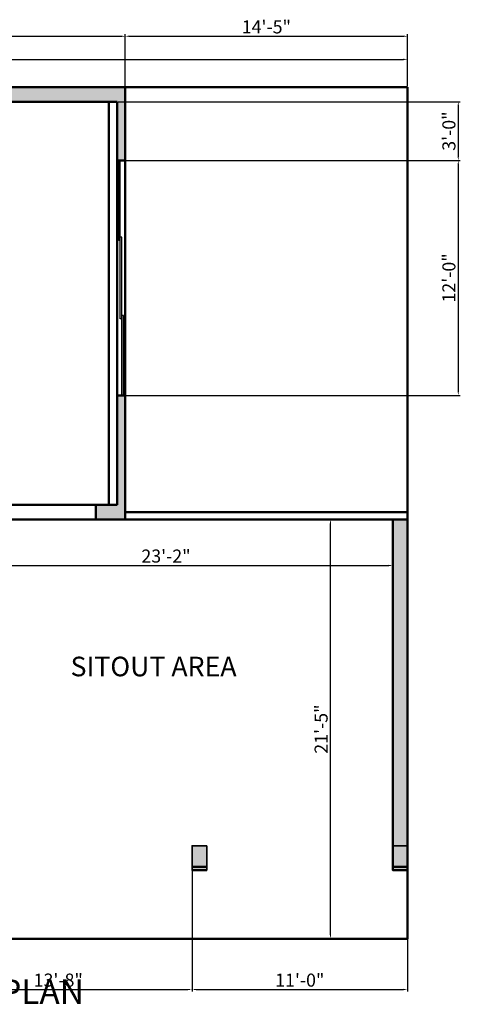
# Model space of a CAD drawing. Units: inches. Extents: x 1770 to 3141, y 984 to 1614.
# Tile 12 of 12: x 2871 to 3141, y 1003 to 1606. Entities that reach past the tile are written whole.
import ezdxf

# ---------------------------------------------------------------- set-up
doc = ezdxf.new("R2010")
doc.units = ezdxf.units.IN
for name, color, linetype, lineweight in [('A-ANNO-DIMS', 2, 'Continuous', 18), ('A-ANNO-TEXT', 7, 'Continuous', 18), ('A-AREA-IDEN', 3, 'Continuous', 18), ('A-COLS', 1, 'Continuous', 35), ('A-GLAZ', 5, 'Continuous', 25), ('A-WALL', 7, 'Continuous', 50), ('A-WALL-PATT', 8, 'Continuous', 13)]:
    doc.layers.add(name, color=color, linetype=linetype, lineweight=lineweight)
doc.styles.get("Standard").update_dxf_attribs({"font": 'arial.ttf'})
doc.dimstyles.new('ISO-25', dxfattribs={"dimtxt": 8, "dimasz": 2.5, "dimexe": 1.25, "dimexo": 0.625, "dimtad": 1, "dimdec": 1, "dimlunit": 3, "dimtxsty": 'Standard', "dimcen": 2.5, "dimclrt": 1, "dimadec": 0, "dimazin": 0, "dimtfac": 1, "dimtdec": 1, "dimtmove": 0, "dimatfit": 3, "dimfxl": 1, "dimarcsym": 0})

# ---------------------------------------------------------------- blocks, each defined once
blk = doc.blocks.new('*D20')
at = {"layer": 'A-ANNO-DIMS', "color": 0, "lineweight": -2, "transparency": 16777216}
for p, q in [((2509.08, 1565.8), (2509.08, 1583.37)), ((2511.58, 1582.12), (3106.58, 1582.12)), ((3109.08, 1565.8), (3109.08, 1583.37))]:
    blk.add_line(p, q, dxfattribs=at)
at = {"layer": 'A-ANNO-DIMS', "color": 0, "transparency": 16777216}
for points in [[(2511.58, 1582.54), (2511.58, 1581.7), (2509.08, 1582.12)], [(3106.58, 1582.54), (3106.58, 1581.7), (3109.08, 1582.12)]]:
    blk.add_solid(points, dxfattribs=at)
at = {"layer": 'Defpoints', "color": 0, "transparency": 16777216}
for p in [(3109.08, 1582.12), (2509.08, 1565.18), (3109.08, 1565.18)]:
    blk.add_point(p, dxfattribs=at)
at = {"layer": 'A-ANNO-DIMS', "color": 0, "transparency": 16777216, "insert": (2809.08, 1586.83), "char_height": 8, "attachment_point": 5}
blk.add_mtext("50'", dxfattribs=at)
blk = doc.blocks.new('*D52')
at = {"layer": 'A-ANNO-DIMS', "color": 0, "lineweight": -2, "transparency": 16777216}
for p, q in [((2822.08, 1274.4), (2822.08, 1270.71)), ((3100.08, 1274.4), (3100.08, 1270.71)), ((2824.58, 1271.96), (3097.58, 1271.96))]:
    blk.add_line(p, q, dxfattribs=at)
at = {"layer": 'A-ANNO-DIMS', "color": 0, "transparency": 16777216}
for points in [[(2824.58, 1272.38), (2824.58, 1271.54), (2822.08, 1271.96)], [(3097.58, 1272.38), (3097.58, 1271.54), (3100.08, 1271.96)]]:
    blk.add_solid(points, dxfattribs=at)
at = {"layer": 'Defpoints', "color": 0, "transparency": 16777216}
for p in [(2822.08, 1275.03), (3100.08, 1275.03), (3100.08, 1271.96)]:
    blk.add_point(p, dxfattribs=at)
at = {"layer": 'A-ANNO-DIMS', "color": 0, "transparency": 16777216, "insert": (2961.08, 1276.67), "char_height": 8, "attachment_point": 5}
blk.add_mtext('23\'-2"', dxfattribs=at)
blk = doc.blocks.new('*D53')
at = {"layer": 'A-ANNO-DIMS', "color": 0, "lineweight": -2, "transparency": 16777216}
for p, q in [((3061.88, 1045.68), (3061.88, 1297.68)), ((3062.5, 1300.18), (3063.13, 1300.18)), ((3062.5, 1043.18), (3063.13, 1043.18))]:
    blk.add_line(p, q, dxfattribs=at)
at = {"layer": 'A-ANNO-DIMS', "color": 0, "transparency": 16777216}
for points in [[(3061.46, 1297.68), (3062.29, 1297.68), (3061.88, 1300.18)], [(3061.46, 1045.68), (3062.29, 1045.68), (3061.88, 1043.18)]]:
    blk.add_solid(points, dxfattribs=at)
at = {"layer": 'Defpoints', "color": 0, "transparency": 16777216}
for p in [(3061.88, 1300.18), (3061.88, 1300.18), (3061.88, 1043.18)]:
    blk.add_point(p, dxfattribs=at)
at = {"layer": 'A-ANNO-DIMS', "color": 0, "transparency": 16777216, "insert": (3057.17, 1171.68), "char_height": 8, "attachment_point": 5, "rotation": 90}
blk.add_mtext('21\'-5"', dxfattribs=at)
blk = doc.blocks.new('COLUMN-9x15')
at = {"transparency": 33554687}
h = blk.add_hatch(color=256, dxfattribs=at)
h.dxf.hatch_style = 1
h.paths.add_polyline_path([(9, 15), (0, 15), (0, 0), (9, 0)])
blk.add_lwpolyline([(9, 15), (0, 15), (0, 0), (9, 0)], close=True)
blk = doc.blocks.new('*D124')
at = {"layer": 'A-ANNO-DIMS', "color": 0, "lineweight": -2, "transparency": 16777216}
for p, q in [((2735.08, 1556.8), (2735.08, 1597.53)), ((2737.58, 1596.28), (2933.58, 1596.28)), ((2936.08, 1565.8), (2936.08, 1597.53))]:
    blk.add_line(p, q, dxfattribs=at)
at = {"layer": 'A-ANNO-DIMS', "color": 0, "transparency": 16777216}
for points in [[(2737.58, 1596.7), (2737.58, 1595.86), (2735.08, 1596.28)], [(2933.58, 1596.7), (2933.58, 1595.86), (2936.08, 1596.28)]]:
    blk.add_solid(points, dxfattribs=at)
at = {"layer": 'Defpoints', "color": 0, "transparency": 16777216}
for p in [(2936.08, 1596.28), (2936.08, 1565.18), (2735.08, 1556.18)]:
    blk.add_point(p, dxfattribs=at)
at = {"layer": 'A-ANNO-DIMS', "color": 1, "transparency": 16777216, "insert": (2835.58, 1600.99), "char_height": 8, "attachment_point": 5}
blk.add_mtext('16\'-9"', dxfattribs=at)
blk = doc.blocks.new('*D125')
at = {"layer": 'A-ANNO-DIMS', "color": 0, "lineweight": -2, "transparency": 16777216}
for p, q in [((2936.08, 1565.8), (2936.08, 1597.53)), ((2938.58, 1596.28), (3106.58, 1596.28)), ((3109.08, 1565.8), (3109.08, 1597.53))]:
    blk.add_line(p, q, dxfattribs=at)
at = {"layer": 'A-ANNO-DIMS', "color": 0, "transparency": 16777216}
for points in [[(2938.58, 1596.7), (2938.58, 1595.86), (2936.08, 1596.28)], [(3106.58, 1596.7), (3106.58, 1595.86), (3109.08, 1596.28)]]:
    blk.add_solid(points, dxfattribs=at)
at = {"layer": 'Defpoints', "color": 0, "transparency": 16777216}
for p in [(3109.08, 1596.28), (2936.08, 1565.18), (3109.08, 1565.18)]:
    blk.add_point(p, dxfattribs=at)
at = {"layer": 'A-ANNO-DIMS', "color": 1, "transparency": 16777216, "insert": (3022.58, 1600.99), "char_height": 8, "attachment_point": 5}
blk.add_mtext('14\'-5"', dxfattribs=at)
blk = doc.blocks.new('*D133')
at = {"layer": 'A-ANNO-DIMS', "color": 0, "lineweight": -2, "transparency": 16777216}
for p, q in [((2813.08, 1084.55), (2813.08, 1010.83)), ((2977.04, 1084.55), (2977.04, 1010.83)), ((2815.58, 1012.08), (2974.54, 1012.08))]:
    blk.add_line(p, q, dxfattribs=at)
at = {"layer": 'A-ANNO-DIMS', "color": 0, "transparency": 16777216}
for points in [[(2815.58, 1012.5), (2815.58, 1011.66), (2813.08, 1012.08)], [(2974.54, 1012.5), (2974.54, 1011.66), (2977.04, 1012.08)]]:
    blk.add_solid(points, dxfattribs=at)
at = {"layer": 'Defpoints', "color": 0, "transparency": 16777216}
for p in [(2813.08, 1085.18), (2977.04, 1085.18), (2977.04, 1012.08)]:
    blk.add_point(p, dxfattribs=at)
at = {"layer": 'A-ANNO-DIMS', "color": 1, "transparency": 16777216, "insert": (2895.06, 1016.79), "char_height": 8, "attachment_point": 5}
blk.add_mtext('13\'-8"', dxfattribs=at)
blk = doc.blocks.new('*D134')
at = {"layer": 'A-ANNO-DIMS', "color": 0, "lineweight": -2, "transparency": 16777216}
for p, q in [((2977.04, 1084.55), (2977.04, 1010.83)), ((3109.08, 1084.55), (3109.08, 1010.83)), ((2979.54, 1012.08), (3106.58, 1012.08))]:
    blk.add_line(p, q, dxfattribs=at)
at = {"layer": 'A-ANNO-DIMS', "color": 0, "transparency": 16777216}
for points in [[(2979.54, 1012.5), (2979.54, 1011.66), (2977.04, 1012.08)], [(3106.58, 1012.5), (3106.58, 1011.66), (3109.08, 1012.08)]]:
    blk.add_solid(points, dxfattribs=at)
at = {"layer": 'Defpoints', "color": 0, "transparency": 16777216}
for p in [(2977.04, 1085.18), (3109.08, 1085.18), (3109.08, 1012.08)]:
    blk.add_point(p, dxfattribs=at)
at = {"layer": 'A-ANNO-DIMS', "color": 1, "transparency": 16777216, "insert": (3043.06, 1016.79), "char_height": 8, "attachment_point": 5}
blk.add_mtext('11\'-0"', dxfattribs=at)
blk = doc.blocks.new('*D138')
at = {"layer": 'A-ANNO-DIMS', "color": 0, "lineweight": -2, "transparency": 16777216}
for p, q in [((2931.7, 1556.18), (3141.43, 1556.18)), ((3140.18, 1553.68), (3140.18, 1522.68)), ((2933.7, 1520.18), (3141.43, 1520.18))]:
    blk.add_line(p, q, dxfattribs=at)
at = {"layer": 'A-ANNO-DIMS', "color": 0, "transparency": 16777216}
for points in [[(3139.76, 1553.68), (3140.6, 1553.68), (3140.18, 1556.18)], [(3139.76, 1522.68), (3140.6, 1522.68), (3140.18, 1520.18)]]:
    blk.add_solid(points, dxfattribs=at)
at = {"layer": 'Defpoints', "color": 0, "transparency": 16777216}
for p in [(2931.08, 1556.18), (2933.08, 1520.18), (3140.18, 1520.18)]:
    blk.add_point(p, dxfattribs=at)
at = {"layer": 'A-ANNO-DIMS', "color": 1, "transparency": 16777216, "insert": (3135.47, 1538.18), "char_height": 8, "attachment_point": 5, "rotation": 90}
blk.add_mtext('3\'-0"', dxfattribs=at)
blk = doc.blocks.new('*D139')
at = {"layer": 'A-ANNO-DIMS', "color": 0, "lineweight": -2, "transparency": 16777216}
for p, q in [((2933.7, 1520.18), (3141.43, 1520.18)), ((3140.18, 1517.68), (3140.18, 1378.68)), ((2934.7, 1376.18), (3141.43, 1376.18))]:
    blk.add_line(p, q, dxfattribs=at)
at = {"layer": 'A-ANNO-DIMS', "color": 0, "transparency": 16777216}
for points in [[(3139.76, 1517.68), (3140.6, 1517.68), (3140.18, 1520.18)], [(3139.76, 1378.68), (3140.6, 1378.68), (3140.18, 1376.18)]]:
    blk.add_solid(points, dxfattribs=at)
at = {"layer": 'Defpoints', "color": 0, "transparency": 16777216}
for p in [(2933.08, 1520.18), (2934.08, 1376.18), (3140.18, 1376.18)]:
    blk.add_point(p, dxfattribs=at)
at = {"layer": 'A-ANNO-DIMS', "color": 1, "transparency": 16777216, "insert": (3135.47, 1448.18), "char_height": 8, "attachment_point": 5, "rotation": 90}
blk.add_mtext('12\'-0"', dxfattribs=at)

msp = doc.modelspace()

# ---------------------------------------------------------------- hatches: boundary and pattern name
at = {"layer": 'A-WALL-PATT'}
h = msp.add_hatch(color=256, dxfattribs=at)
h.dxf.hatch_style = 1
h.paths.add_polyline_path([(2936.08, 1565.18), (2509.08, 1565.18), (2509.08, 1100.18), (2518.08, 1100.18), (2518.08, 1125.25), (2518.08, 1246.18), (2662.08, 1246.18), (2662.08, 1251.18), (2518.08, 1251.18), (2518.08, 1407.18), (2641.08, 1407.18), (2641.08, 1412.18), (2518.08, 1412.18), (2518.08, 1556.18), (2540.6, 1556.18), (2931.08, 1556.18), (2931.08, 1520.18), (2936.08, 1520.18)])
h.paths.add_polyline_path([(2560.08, 1094.18), (2518.08, 1094.18), (2518.08, 1085.18), (2560.08, 1085.18)])
h.paths.add_polyline_path([(2662.08, 1094.18), (2620.08, 1094.18), (2620.08, 1085.18), (2662.08, 1085.18)])
h.paths.add_polyline_path([(2783.08, 1094.18), (2707.08, 1094.18), (2707.08, 1085.18), (2783.08, 1085.18)])
h.paths.add_polyline_path([(2703.08, 1179.18), (2698.08, 1179.18), (2698.08, 1100.18), (2703.08, 1100.18)], flags=16)
h.paths.add_polyline_path([(2813.08, 1094.18), (2807.08, 1094.18), (2807.08, 1085.18), (2813.08, 1085.18)])
h.paths.add_polyline_path([(2822.08, 1300.18), (2834.08, 1300.18), (2834.08, 1309.18), (2813.08, 1309.18), (2813.08, 1251.18), (2698.08, 1251.18), (2698.08, 1215.18), (2698.08, 1209.18), (2703.08, 1209.18), (2703.08, 1246.18), (2813.08, 1246.18), (2813.08, 1167.18), (2733.08, 1167.18), (2733.08, 1162.18), (2813.08, 1162.18), (2813.08, 1100.18), (2822.08, 1100.18)], flags=17)
h.paths.add_polyline_path([(2936.08, 1376.18), (2931.08, 1376.18), (2931.08, 1309.18), (2918.08, 1309.18), (2918.08, 1300.18), (2936.08, 1300.18)], flags=17)
h.paths.add_polyline_path([(2735.08, 1520.18), (2718.08, 1520.18), (2718.08, 1515.18), (2730.08, 1515.18), (2730.08, 1412.18), (2682.08, 1412.18), (2682.08, 1448.18), (2677.08, 1448.18), (2677.08, 1407.18), (2735.08, 1407.18)], flags=17)
h.paths.add_polyline_path([(2682.08, 1515.18), (2694.08, 1515.18), (2694.08, 1520.18), (2677.08, 1520.18), (2677.08, 1478.18), (2682.08, 1478.18)], flags=16)
h = msp.add_hatch(color=256, dxfattribs=at)
h.dxf.hatch_style = 1
h.paths.add_polyline_path([(3109.08, 1300.18), (3100.08, 1300.18), (3100.08, 1100.18), (3109.08, 1100.18)])

# ---------------------------------------------------------------- linework, layer by layer
at = {"layer": 'A-GLAZ'}
for p, q in [((2932.08, 1471.18), (2932.08, 1520.18)), ((2933.08, 1423.18), (2933.08, 1520.18)), ((2934.08, 1473.18), (2933.08, 1473.18)), ((2934.08, 1376.18), (2934.08, 1473.18)), ((2933.08, 1471.18), (2932.08, 1471.18)), ((2935.08, 1425.18), (2934.08, 1425.18)), ((2935.08, 1376.18), (2935.08, 1425.18)), ((2934.08, 1423.18), (2933.08, 1423.18))]:
    msp.add_line(p, q, dxfattribs=at)
at = {"layer": 'A-WALL'}
for p, q in [((2509.08, 1565.18), (3109.08, 1565.18)), ((2936.08, 1565.18), (2936.08, 1300.18)), ((3109.08, 1565.18), (3109.08, 1043.18)), ((2518.08, 1556.18), (2931.08, 1556.18)), ((2926.08, 1556.18), (2926.08, 1309.18)), ((2931.08, 1556.18), (2931.08, 1309.18)), ((2931.08, 1520.18), (2936.08, 1520.18)), ((2931.08, 1376.18), (2936.08, 1376.18)), ((2918.08, 1309.18), (2834.08, 1309.18)), ((2918.08, 1300.18), (2918.08, 1309.18)), ((2918.08, 1309.18), (2931.08, 1309.18)), ((2936.08, 1304.68), (3109.08, 1304.68)), ((2918.08, 1300.18), (2834.08, 1300.18)), ((2918.08, 1300.18), (3109.08, 1300.18)), ((3100.08, 1300.18), (3100.08, 1085.18)), ((2986.04, 1087.18), (2977.04, 1087.18)), ((3109.08, 1087.18), (3100.08, 1087.18)), ((2986.04, 1085.18), (2977.04, 1085.18)), ((3109.08, 1085.18), (3100.08, 1085.18)), ((3109.08, 1043.18), (2509.08, 1043.18))]:
    msp.add_line(p, q, dxfattribs=at)

# ---------------------------------------------------------------- block references
at = {"layer": 'A-COLS'}
for p in [(2977.04, 1085.18), (3100.08, 1085.18)]:
    msp.add_blockref('COLUMN-9x15', p, dxfattribs=at)

# ---------------------------------------------------------------- texts
at = {"layer": 'A-ANNO-TEXT', "insert": (2729.78, 1018.27), "char_height": 15, "attachment_point": 1}
msp.add_mtext_dynamic_manual_height_columns('FIRST FLOOR PLAN', width=253.2094, gutter_width=12.5, heights=[0], dxfattribs=at)
at = {"layer": 'A-AREA-IDEN', "insert": (2902.6, 1216.04), "char_height": 12, "attachment_point": 1}
msp.add_mtext_dynamic_manual_height_columns('SITOUT AREA', width=159.3747, gutter_width=12.5, heights=[0], dxfattribs=at)

# ---------------------------------------------------------------- dimensions: what is measured, and where the dimension line sits
at = {"layer": 'A-ANNO-DIMS'}
for base, p1, p2, override, picture, middle in [((2936.08, 1596.28), (2735.08, 1556.18), (2936.08, 1565.18), {"dimdec": 1, "dimlfac": 1, "dimrnd": 0, "dimzin": 1, "dimdsep": 46, "dimlunit": 4, "dimfrac": 2}, '*D124', (2835.58, 1600.99)), ((3109.08, 1596.28), (2936.08, 1565.18), (3109.08, 1565.18), {"dimdec": 1, "dimlfac": 1, "dimrnd": 0, "dimzin": 1, "dimdsep": 46, "dimlunit": 4, "dimfrac": 2}, '*D125', (3022.58, 1600.99)), ((3109.08, 1582.12), (2509.08, 1565.18), (3109.08, 1565.18), {"dimclrd": 0, "dimclre": 0, "dimclrt": 0}, '*D20', (2809.08, 1586.83)), ((3100.08, 1271.96), (2822.08, 1275.03), (3100.08, 1275.03), {"dimclrd": 0, "dimclre": 0, "dimclrt": 0}, '*D52', (2961.08, 1276.67)), ((2977.04, 1012.08), (2813.08, 1085.18), (2977.04, 1085.18), {"dimdec": 1, "dimlfac": 1, "dimrnd": 0, "dimzin": 1, "dimdsep": 46, "dimlunit": 4, "dimfrac": 2}, '*D133', (2895.06, 1016.79)), ((3109.08, 1012.08), (2977.04, 1085.18), (3109.08, 1085.18), {"dimdec": 1, "dimlfac": 1, "dimrnd": 0, "dimzin": 1, "dimdsep": 46, "dimlunit": 4, "dimfrac": 2}, '*D134', (3043.06, 1016.79))]:
    dim = msp.add_linear_dim(base=base, p1=p1, p2=p2, dimstyle='ISO-25', override=override, dxfattribs=at)
    dim.commit()
    dim.dimension.update_dxf_attribs({"geometry": picture, "text_midpoint": middle})
for base, p1, p2, override, picture, middle in [((3140.18, 1520.18), (2931.08, 1556.18), (2933.08, 1520.18), {"dimdec": 1, "dimlfac": 1, "dimrnd": 0, "dimzin": 1, "dimdsep": 46, "dimlunit": 4, "dimfrac": 2}, '*D138', (3135.47, 1538.18)), ((3140.18, 1376.18), (2933.08, 1520.18), (2934.08, 1376.18), {"dimdec": 1, "dimlfac": 1, "dimrnd": 0, "dimzin": 1, "dimdsep": 46, "dimlunit": 4, "dimfrac": 2}, '*D139', (3135.47, 1448.18)), ((3061.88, 1300.18), (3061.88, 1043.18), (3061.88, 1300.18), {"dimclrd": 0, "dimclre": 0, "dimclrt": 0}, '*D53', (3057.17, 1171.68))]:
    dim = msp.add_linear_dim(base=base, p1=p1, p2=p2, angle=90, dimstyle='ISO-25', override=override, dxfattribs=at)
    dim.commit()
    dim.dimension.update_dxf_attribs({"geometry": picture, "text_midpoint": middle})

doc.saveas('drawing.dxf')
